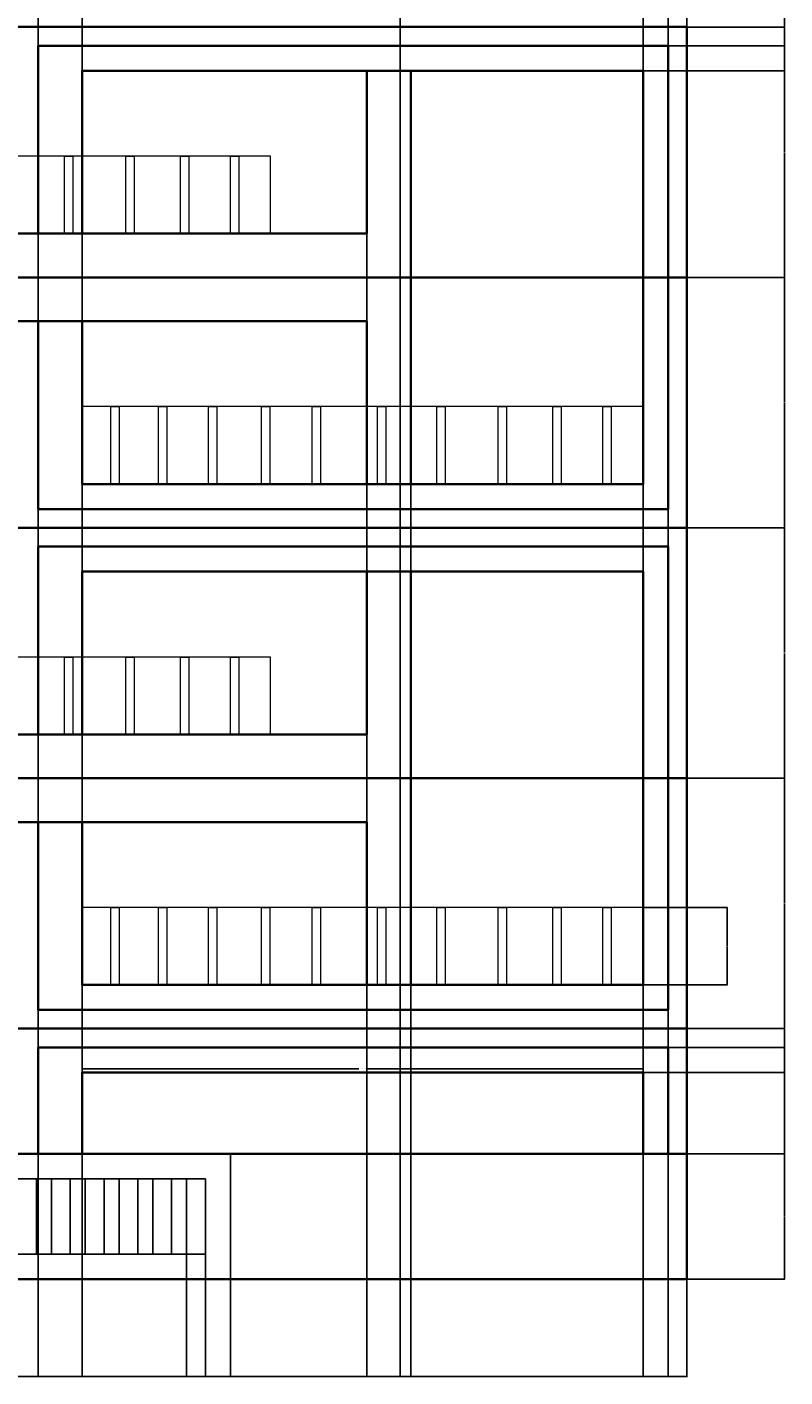
# Model space of a CAD drawing. Units: inches. Extents: x -26 to 668, y -42 to 976.
# Tile 2 of 3: x 305 to 668, y -42 to 605. Entities that reach past the tile are written whole.
import ezdxf

# ---------------------------------------------------------------- set-up
doc = ezdxf.new("R2010")
doc.units = ezdxf.units.IN
doc.header["$MEASUREMENT"] = 0
for name, color, linetype, lineweight in [('A-ANNO-DIMS', 2, 'Continuous', 18), ('A-DOOR', 3, 'Continuous', 25), ('A-ELEV', 7, 'Continuous', 35), ('A-FLOR-HRAL', 8, 'Continuous', 18)]:
    doc.layers.add(name, color=color, linetype=linetype, lineweight=lineweight)
doc.styles.get("Standard").update_dxf_attribs({"font": 'arial.ttf'})
doc.dimstyles.get("Standard").update_dxf_attribs({"dimtxt": 0.18, "dimasz": 0.18, "dimexe": 0.18, "dimexo": 0.0625, "dimgap": 0.09, "dimtad": 0, "dimtih": 1, "dimtoh": 1, "dimdec": 4, "dimzin": 0, "dimdsep": 46, "dimtxsty": 'Standard', "dimcen": 0.09, "dimadec": 0, "dimazin": 0, "dimtfac": 1, "dimtdec": 4, "dimtofl": 0, "dimtmove": 0, "dimatfit": 3, "dimfxl": 1, "dimtolj": 1, "dimtzin": 0, "dimarcsym": 0})

# ---------------------------------------------------------------- blocks, each defined once
blk = doc.blocks.new('RAILING-BALCONY')
for points in [[(331.17, 145.96), (599.79, 145.96), (599.79, 183.06), (331.17, 183.06)], [(344.86, 183.06), (348.85, 183.06), (348.85, 145.96), (344.86, 145.96)], [(367.74, 183.06), (371.72, 183.06), (371.72, 145.96), (367.74, 145.96)], [(391.66, 183.06), (395.64, 183.06), (395.64, 145.96), (391.66, 145.96)], [(417.04, 183.06), (421.03, 183.06), (421.03, 145.96), (417.04, 145.96)], [(441.38, 183.06), (445.37, 183.06), (445.37, 145.96), (441.38, 145.96)], [(472.69, 183.06), (476.68, 183.06), (476.68, 145.96), (472.69, 145.96)], [(501.02, 183.06), (505, 183.06), (505, 145.96), (501.02, 145.96)], [(530.39, 183.06), (534.38, 183.06), (534.38, 145.96), (530.39, 145.96)], [(556.62, 183.06), (560.61, 183.06), (560.61, 145.96), (556.62, 145.96)], [(580.54, 183.06), (584.53, 183.06), (584.53, 145.96), (580.54, 145.96)]]:
    blk.add_lwpolyline(points, close=True)
blk = doc.blocks.new('*D3')
at = {"layer": 'A-ANNO-DIMS', "color": 0, "lineweight": -2, "transparency": 16777216}
for p, q in [((331.17, 145.9), (331.17, 105.49)), ((599.79, 145.9), (599.79, 105.49)), ((331.35, 105.67), (463.72, 105.67)), ((599.61, 105.67), (467.25, 105.67))]:
    blk.add_line(p, q, dxfattribs=at)
at = {"layer": 'A-ANNO-DIMS', "color": 0, "transparency": 16777216}
for points in [[(331.35, 105.7), (331.35, 105.64), (331.17, 105.67)], [(599.61, 105.7), (599.61, 105.64), (599.79, 105.67)]]:
    blk.add_solid(points, dxfattribs=at)
at = {"layer": 'Defpoints', "color": 0, "transparency": 16777216}
for p in [(331.17, 145.96), (599.79, 145.96), (599.79, 105.67)]:
    blk.add_point(p, dxfattribs=at)
at = {"layer": 'A-ANNO-DIMS', "color": 0, "transparency": 16777216, "insert": (465.48, 105.67), "char_height": 0.18, "attachment_point": 5}
blk.add_mtext('\\A1;BALCONY RAILING 269 TYP.', dxfattribs=at)
blk = doc.blocks.new('*D4')
at = {"layer": 'A-ANNO-DIMS', "color": 0, "lineweight": -2, "transparency": 16777216}
for p, q in [((599.86, 183.06), (640.27, 183.06)), ((640.09, 182.88), (640.09, 164.69)), ((640.09, 146.14), (640.09, 164.33)), ((599.86, 145.96), (640.27, 145.96))]:
    blk.add_line(p, q, dxfattribs=at)
at = {"layer": 'A-ANNO-DIMS', "color": 0, "transparency": 16777216}
for points in [[(640.06, 182.88), (640.12, 182.88), (640.09, 183.06)], [(640.06, 146.14), (640.12, 146.14), (640.09, 145.96)]]:
    blk.add_solid(points, dxfattribs=at)
at = {"layer": 'Defpoints', "color": 0, "transparency": 16777216}
for p in [(599.79, 183.06), (640.09, 183.06), (599.79, 145.96)]:
    blk.add_point(p, dxfattribs=at)
at = {"layer": 'A-ANNO-DIMS', "color": 0, "transparency": 16777216, "insert": (640.09, 164.51), "char_height": 0.18, "attachment_point": 5}
blk.add_mtext('\\A1;37 TYP.', dxfattribs=at)
blk = doc.blocks.new('*D9')
at = {"layer": 'A-ANNO-DIMS', "color": 0, "lineweight": -2, "transparency": 16777216}
for p, q in [((620.86, 124.96), (667.72, 124.96)), ((667.54, 124.78), (667.54, 95.14)), ((667.54, 65.14), (667.54, 94.78)), ((620.86, 64.96), (667.72, 64.96))]:
    blk.add_line(p, q, dxfattribs=at)
at = {"layer": 'A-ANNO-DIMS', "color": 0, "transparency": 16777216}
for points in [[(667.51, 124.78), (667.57, 124.78), (667.54, 124.96)], [(667.51, 65.14), (667.57, 65.14), (667.54, 64.96)]]:
    blk.add_solid(points, dxfattribs=at)
at = {"layer": 'Defpoints', "color": 0, "transparency": 16777216}
for p in [(620.79, 124.96), (667.54, 124.96), (620.79, 64.96)]:
    blk.add_point(p, dxfattribs=at)
at = {"layer": 'A-ANNO-DIMS', "color": 0, "transparency": 16777216, "insert": (667.54, 94.96), "char_height": 0.18, "attachment_point": 5}
blk.add_mtext('\\A1;60', dxfattribs=at)
blk = doc.blocks.new('*D10')
at = {"layer": 'A-ANNO-DIMS', "color": 0, "lineweight": -2, "transparency": 16777216}
for p, q in [((620.86, 244.96), (667.72, 244.96)), ((667.54, 244.78), (667.54, 185.14)), ((667.54, 125.14), (667.54, 184.78)), ((620.86, 124.96), (667.72, 124.96))]:
    blk.add_line(p, q, dxfattribs=at)
at = {"layer": 'A-ANNO-DIMS', "color": 0, "transparency": 16777216}
for points in [[(667.51, 244.78), (667.57, 244.78), (667.54, 244.96)], [(667.51, 125.14), (667.57, 125.14), (667.54, 124.96)]]:
    blk.add_solid(points, dxfattribs=at)
at = {"layer": 'Defpoints', "color": 0, "transparency": 16777216}
for p in [(620.79, 244.96), (667.54, 244.96), (620.79, 124.96)]:
    blk.add_point(p, dxfattribs=at)
at = {"layer": 'A-ANNO-DIMS', "color": 0, "transparency": 16777216, "insert": (667.54, 184.96), "char_height": 0.18, "attachment_point": 5}
blk.add_mtext('\\A1;120', dxfattribs=at)
blk = doc.blocks.new('*D11')
at = {"layer": 'A-ANNO-DIMS', "color": 0, "lineweight": -2, "transparency": 16777216}
for p, q in [((620.86, 364.96), (667.72, 364.96)), ((667.54, 364.78), (667.54, 305.14)), ((667.54, 245.14), (667.54, 304.78)), ((620.86, 244.96), (667.72, 244.96))]:
    blk.add_line(p, q, dxfattribs=at)
at = {"layer": 'A-ANNO-DIMS', "color": 0, "transparency": 16777216}
for points in [[(667.51, 364.78), (667.57, 364.78), (667.54, 364.96)], [(667.51, 245.14), (667.57, 245.14), (667.54, 244.96)]]:
    blk.add_solid(points, dxfattribs=at)
at = {"layer": 'Defpoints', "color": 0, "transparency": 16777216}
for p in [(620.79, 364.96), (667.54, 364.96), (620.79, 244.96)]:
    blk.add_point(p, dxfattribs=at)
at = {"layer": 'A-ANNO-DIMS', "color": 0, "transparency": 16777216, "insert": (667.54, 304.96), "char_height": 0.18, "attachment_point": 5}
blk.add_mtext('\\A1;120', dxfattribs=at)
blk = doc.blocks.new('*D12')
at = {"layer": 'A-ANNO-DIMS', "color": 0, "lineweight": -2, "transparency": 16777216}
for p, q in [((620.86, 484.96), (667.72, 484.96)), ((667.54, 484.78), (667.54, 425.14)), ((667.54, 365.14), (667.54, 424.78)), ((620.86, 364.96), (667.72, 364.96))]:
    blk.add_line(p, q, dxfattribs=at)
at = {"layer": 'A-ANNO-DIMS', "color": 0, "transparency": 16777216}
for points in [[(667.51, 484.78), (667.57, 484.78), (667.54, 484.96)], [(667.51, 365.14), (667.57, 365.14), (667.54, 364.96)]]:
    blk.add_solid(points, dxfattribs=at)
at = {"layer": 'Defpoints', "color": 0, "transparency": 16777216}
for p in [(620.79, 484.96), (667.54, 484.96), (620.79, 364.96)]:
    blk.add_point(p, dxfattribs=at)
at = {"layer": 'A-ANNO-DIMS', "color": 0, "transparency": 16777216, "insert": (667.54, 424.96), "char_height": 0.18, "attachment_point": 5}
blk.add_mtext('\\A1;120', dxfattribs=at)
blk = doc.blocks.new('*D13')
at = {"layer": 'A-ANNO-DIMS', "color": 0, "lineweight": -2, "transparency": 16777216}
for p, q in [((620.86, 604.96), (667.72, 604.96)), ((667.54, 604.78), (667.54, 545.14)), ((667.54, 485.14), (667.54, 544.78)), ((620.86, 484.96), (667.72, 484.96))]:
    blk.add_line(p, q, dxfattribs=at)
at = {"layer": 'A-ANNO-DIMS', "color": 0, "transparency": 16777216}
for points in [[(667.51, 604.78), (667.57, 604.78), (667.54, 604.96)], [(667.51, 485.14), (667.57, 485.14), (667.54, 484.96)]]:
    blk.add_solid(points, dxfattribs=at)
at = {"layer": 'Defpoints', "color": 0, "transparency": 16777216}
for p in [(620.79, 604.96), (667.54, 604.96), (620.79, 484.96)]:
    blk.add_point(p, dxfattribs=at)
at = {"layer": 'A-ANNO-DIMS', "color": 0, "transparency": 16777216, "insert": (667.54, 544.96), "char_height": 0.18, "attachment_point": 5}
blk.add_mtext('\\A1;120', dxfattribs=at)
blk = doc.blocks.new('*D14')
at = {"layer": 'A-ANNO-DIMS', "color": 0, "lineweight": -2, "transparency": 16777216}
for p, q in [((620.86, 724.96), (667.72, 724.96)), ((667.54, 724.78), (667.54, 665.14)), ((667.54, 605.14), (667.54, 664.78)), ((620.86, 604.96), (667.72, 604.96))]:
    blk.add_line(p, q, dxfattribs=at)
at = {"layer": 'A-ANNO-DIMS', "color": 0, "transparency": 16777216}
for points in [[(667.51, 724.78), (667.57, 724.78), (667.54, 724.96)], [(667.51, 605.14), (667.57, 605.14), (667.54, 604.96)]]:
    blk.add_solid(points, dxfattribs=at)
at = {"layer": 'Defpoints', "color": 0, "transparency": 16777216}
for p in [(620.79, 724.96), (667.54, 724.96), (620.79, 604.96)]:
    blk.add_point(p, dxfattribs=at)
at = {"layer": 'A-ANNO-DIMS', "color": 0, "transparency": 16777216, "insert": (667.54, 664.96), "char_height": 0.18, "attachment_point": 5}
blk.add_mtext('\\A1;120', dxfattribs=at)
blk = doc.blocks.new('*D22')
at = {"layer": 'A-ANNO-DIMS', "color": 0, "lineweight": -2, "transparency": 16777216}
for p, q in [((140.65, 844.9), (140.65, -41.97)), ((483.43, 844.9), (483.43, -41.97)), ((140.83, -41.79), (311.65, -41.79)), ((483.25, -41.79), (312.43, -41.79))]:
    blk.add_line(p, q, dxfattribs=at)
at = {"layer": 'A-ANNO-DIMS', "color": 0, "transparency": 16777216}
for points in [[(140.83, -41.76), (140.83, -41.82), (140.65, -41.79)], [(483.25, -41.76), (483.25, -41.82), (483.43, -41.79)]]:
    blk.add_solid(points, dxfattribs=at)
at = {"layer": 'Defpoints', "color": 0, "transparency": 16777216}
for p in [(140.65, 844.96), (483.43, 844.96), (483.43, -41.79)]:
    blk.add_point(p, dxfattribs=at)
at = {"layer": 'A-ANNO-DIMS', "color": 0, "transparency": 16777216, "insert": (312.04, -41.79), "char_height": 0.18, "attachment_point": 5}
blk.add_mtext('\\A1;342.8', dxfattribs=at)
blk = doc.blocks.new('*D30')
at = {"layer": 'A-ANNO-DIMS', "color": 0, "lineweight": -2, "transparency": 16777216}
for p, q in [((152.83, 505.9), (152.83, -41.97)), ((310.17, 505.9), (310.17, -41.97)), ((153.01, -41.79), (231.05, -41.79)), ((309.99, -41.79), (231.96, -41.79))]:
    blk.add_line(p, q, dxfattribs=at)
at = {"layer": 'A-ANNO-DIMS', "color": 0, "transparency": 16777216}
for points in [[(153.01, -41.76), (153.01, -41.82), (152.83, -41.79)], [(309.99, -41.76), (309.99, -41.82), (310.17, -41.79)]]:
    blk.add_solid(points, dxfattribs=at)
at = {"layer": 'Defpoints', "color": 0, "transparency": 16777216}
for p in [(152.83, 505.96), (310.17, 505.96), (310.17, -41.79)]:
    blk.add_point(p, dxfattribs=at)
at = {"layer": 'A-ANNO-DIMS', "color": 0, "transparency": 16777216, "insert": (231.5, -41.79), "char_height": 0.18, "attachment_point": 5}
blk.add_mtext('\\A1;157.34', dxfattribs=at)
blk = doc.blocks.new('*D31')
at = {"layer": 'A-ANNO-DIMS', "color": 0, "lineweight": -2, "transparency": 16777216}
for p, q in [((310.17, 505.9), (310.17, -41.97)), ((331.17, 505.9), (331.17, -41.97)), ((310.35, -41.79), (320.47, -41.79)), ((330.99, -41.79), (320.87, -41.79))]:
    blk.add_line(p, q, dxfattribs=at)
at = {"layer": 'A-ANNO-DIMS', "color": 0, "transparency": 16777216}
for points in [[(310.35, -41.76), (310.35, -41.82), (310.17, -41.79)], [(330.99, -41.76), (330.99, -41.82), (331.17, -41.79)]]:
    blk.add_solid(points, dxfattribs=at)
at = {"layer": 'Defpoints', "color": 0, "transparency": 16777216}
for p in [(310.17, 505.96), (331.17, 505.96), (331.17, -41.79)]:
    blk.add_point(p, dxfattribs=at)
at = {"layer": 'A-ANNO-DIMS', "color": 0, "transparency": 16777216, "insert": (320.67, -41.79), "char_height": 0.18, "attachment_point": 5}
blk.add_mtext('\\A1;21', dxfattribs=at)
blk = doc.blocks.new('*D32')
at = {"layer": 'A-ANNO-DIMS', "color": 0, "lineweight": -2, "transparency": 16777216}
for p, q in [((331.17, 505.9), (331.17, -41.97)), ((467.51, 505.9), (467.51, -41.97)), ((331.35, -41.79), (398.88, -41.79)), ((467.33, -41.79), (399.79, -41.79))]:
    blk.add_line(p, q, dxfattribs=at)
at = {"layer": 'A-ANNO-DIMS', "color": 0, "transparency": 16777216}
for points in [[(331.35, -41.76), (331.35, -41.82), (331.17, -41.79)], [(467.33, -41.76), (467.33, -41.82), (467.51, -41.79)]]:
    blk.add_solid(points, dxfattribs=at)
at = {"layer": 'Defpoints', "color": 0, "transparency": 16777216}
for p in [(331.17, 505.96), (467.51, 505.96), (467.51, -41.79)]:
    blk.add_point(p, dxfattribs=at)
at = {"layer": 'A-ANNO-DIMS', "color": 0, "transparency": 16777216, "insert": (399.34, -41.79), "char_height": 0.18, "attachment_point": 5}
blk.add_mtext('\\A1;136.34', dxfattribs=at)
blk = doc.blocks.new('*D33')
at = {"layer": 'A-ANNO-DIMS', "color": 0, "lineweight": -2, "transparency": 16777216}
for p, q in [((488.51, 583.9), (488.51, -41.97)), ((467.51, 505.9), (467.51, -41.97)), ((467.69, -41.79), (477.8, -41.79)), ((488.33, -41.79), (478.21, -41.79))]:
    blk.add_line(p, q, dxfattribs=at)
at = {"layer": 'A-ANNO-DIMS', "color": 0, "transparency": 16777216}
for points in [[(467.69, -41.76), (467.69, -41.82), (467.51, -41.79)], [(488.33, -41.76), (488.33, -41.82), (488.51, -41.79)]]:
    blk.add_solid(points, dxfattribs=at)
at = {"layer": 'Defpoints', "color": 0, "transparency": 16777216}
for p in [(488.51, 583.96), (467.51, 505.96), (488.51, -41.79)]:
    blk.add_point(p, dxfattribs=at)
at = {"layer": 'A-ANNO-DIMS', "color": 0, "transparency": 16777216, "insert": (478.01, -41.79), "char_height": 0.18, "attachment_point": 5}
blk.add_mtext('\\A1;21', dxfattribs=at)
blk = doc.blocks.new('*D34')
at = {"layer": 'A-ANNO-DIMS', "color": 0, "lineweight": -2, "transparency": 16777216}
for p, q in [((488.51, 583.9), (488.51, -41.97)), ((599.79, 583.9), (599.79, -41.97)), ((488.69, -41.79), (543.7, -41.79)), ((599.61, -41.79), (544.61, -41.79))]:
    blk.add_line(p, q, dxfattribs=at)
at = {"layer": 'A-ANNO-DIMS', "color": 0, "transparency": 16777216}
for points in [[(488.69, -41.76), (488.69, -41.82), (488.51, -41.79)], [(599.61, -41.76), (599.61, -41.82), (599.79, -41.79)]]:
    blk.add_solid(points, dxfattribs=at)
at = {"layer": 'Defpoints', "color": 0, "transparency": 16777216}
for p in [(488.51, 583.96), (599.79, 583.96), (599.79, -41.79)]:
    blk.add_point(p, dxfattribs=at)
at = {"layer": 'A-ANNO-DIMS', "color": 0, "transparency": 16777216, "insert": (544.15, -41.79), "char_height": 0.18, "attachment_point": 5}
blk.add_mtext('\\A1;111.29', dxfattribs=at)
blk = doc.blocks.new('*D35')
at = {"layer": 'A-ANNO-DIMS', "color": 0, "lineweight": -2, "transparency": 16777216}
for p, q in [((611.79, 595.9), (611.79, -41.97)), ((599.79, 583.9), (599.79, -41.97)), ((599.97, -41.79), (605.58, -41.79)), ((611.61, -41.79), (606, -41.79))]:
    blk.add_line(p, q, dxfattribs=at)
at = {"layer": 'A-ANNO-DIMS', "color": 0, "transparency": 16777216}
for points in [[(599.97, -41.76), (599.97, -41.82), (599.79, -41.79)], [(611.61, -41.76), (611.61, -41.82), (611.79, -41.79)]]:
    blk.add_solid(points, dxfattribs=at)
at = {"layer": 'Defpoints', "color": 0, "transparency": 16777216}
for p in [(611.79, 595.96), (599.79, 583.96), (611.79, -41.79)]:
    blk.add_point(p, dxfattribs=at)
at = {"layer": 'A-ANNO-DIMS', "color": 0, "transparency": 16777216, "insert": (605.79, -41.79), "char_height": 0.18, "attachment_point": 5}
blk.add_mtext('\\A1;12', dxfattribs=at)
blk = doc.blocks.new('*D36')
at = {"layer": 'A-ANNO-DIMS', "color": 0, "lineweight": -2, "transparency": 16777216}
for p, q in [((620.79, 604.9), (620.79, -41.97)), ((611.79, 595.9), (611.79, -41.97)), ((611.97, -41.79), (616.15, -41.79)), ((620.61, -41.79), (616.44, -41.79))]:
    blk.add_line(p, q, dxfattribs=at)
at = {"layer": 'A-ANNO-DIMS', "color": 0, "transparency": 16777216}
for points in [[(611.97, -41.76), (611.97, -41.82), (611.79, -41.79)], [(620.61, -41.76), (620.61, -41.82), (620.79, -41.79)]]:
    blk.add_solid(points, dxfattribs=at)
at = {"layer": 'Defpoints', "color": 0, "transparency": 16777216}
for p in [(620.79, 604.96), (611.79, 595.96), (620.79, -41.79)]:
    blk.add_point(p, dxfattribs=at)
at = {"layer": 'A-ANNO-DIMS', "color": 0, "transparency": 16777216, "insert": (616.29, -41.79), "char_height": 0.18, "attachment_point": 5}
blk.add_mtext('\\A1;9', dxfattribs=at)
blk = doc.blocks.new('*D42')
at = {"layer": 'A-ANNO-DIMS', "color": 0, "lineweight": -2, "transparency": 16777216}
for p, q in [((611.86, 595.96), (667.72, 595.96)), ((667.54, 595.78), (667.54, 590.14)), ((667.54, 584.14), (667.54, 589.78)), ((599.86, 583.96), (667.72, 583.96))]:
    blk.add_line(p, q, dxfattribs=at)
at = {"layer": 'A-ANNO-DIMS', "color": 0, "transparency": 16777216}
for points in [[(667.51, 595.78), (667.57, 595.78), (667.54, 595.96)], [(667.51, 584.14), (667.57, 584.14), (667.54, 583.96)]]:
    blk.add_solid(points, dxfattribs=at)
at = {"layer": 'Defpoints', "color": 0, "transparency": 16777216}
for p in [(611.79, 595.96), (667.54, 595.96), (599.79, 583.96)]:
    blk.add_point(p, dxfattribs=at)
at = {"layer": 'A-ANNO-DIMS', "color": 0, "transparency": 16777216, "insert": (667.54, 589.96), "char_height": 0.18, "attachment_point": 5}
blk.add_mtext('\\A1;12', dxfattribs=at)
blk = doc.blocks.new('*D43')
at = {"layer": 'A-ANNO-DIMS', "color": 0, "lineweight": -2, "transparency": 16777216}
for p, q in [((620.86, 604.96), (667.72, 604.96)), ((667.54, 604.78), (667.54, 600.64)), ((611.86, 595.96), (667.72, 595.96)), ((667.54, 596.14), (667.54, 600.28))]:
    blk.add_line(p, q, dxfattribs=at)
at = {"layer": 'A-ANNO-DIMS', "color": 0, "transparency": 16777216}
for points in [[(667.51, 604.78), (667.57, 604.78), (667.54, 604.96)], [(667.51, 596.14), (667.57, 596.14), (667.54, 595.96)]]:
    blk.add_solid(points, dxfattribs=at)
at = {"layer": 'Defpoints', "color": 0, "transparency": 16777216}
for p in [(620.79, 604.96), (667.54, 604.96), (611.79, 595.96)]:
    blk.add_point(p, dxfattribs=at)
at = {"layer": 'A-ANNO-DIMS', "color": 0, "transparency": 16777216, "insert": (667.54, 600.46), "char_height": 0.18, "attachment_point": 5}
blk.add_mtext('\\A1;9', dxfattribs=at)
blk = doc.blocks.new('*D44')
at = {"layer": 'A-ANNO-DIMS', "color": 0, "lineweight": -2, "transparency": 16777216}
for p, q in [((611.86, 613.96), (667.72, 613.96)), ((667.54, 613.78), (667.54, 609.64)), ((667.54, 605.14), (667.54, 609.28)), ((620.86, 604.96), (667.72, 604.96))]:
    blk.add_line(p, q, dxfattribs=at)
at = {"layer": 'A-ANNO-DIMS', "color": 0, "transparency": 16777216}
for points in [[(667.51, 613.78), (667.57, 613.78), (667.54, 613.96)], [(667.51, 605.14), (667.57, 605.14), (667.54, 604.96)]]:
    blk.add_solid(points, dxfattribs=at)
at = {"layer": 'Defpoints', "color": 0, "transparency": 16777216}
for p in [(611.79, 613.96), (667.54, 613.96), (620.79, 604.96)]:
    blk.add_point(p, dxfattribs=at)
at = {"layer": 'A-ANNO-DIMS', "color": 0, "transparency": 16777216, "insert": (667.54, 609.46), "char_height": 0.18, "attachment_point": 5}
blk.add_mtext('\\A1;9', dxfattribs=at)
blk = doc.blocks.new('*D55')
at = {"layer": 'A-ANNO-DIMS', "color": 0, "lineweight": -2, "transparency": 16777216}
for p, q in [((293.12, 16.9), (293.12, -41.97)), ((381.21, 16.9), (381.21, -41.97)), ((293.3, -41.79), (336.86, -41.79)), ((381.03, -41.79), (337.47, -41.79))]:
    blk.add_line(p, q, dxfattribs=at)
at = {"layer": 'A-ANNO-DIMS', "color": 0, "transparency": 16777216}
for points in [[(293.3, -41.76), (293.3, -41.82), (293.12, -41.79)], [(381.03, -41.76), (381.03, -41.82), (381.21, -41.79)]]:
    blk.add_solid(points, dxfattribs=at)
at = {"layer": 'Defpoints', "color": 0, "transparency": 16777216}
for p in [(293.12, 16.96), (381.21, 16.96), (381.21, -41.79)]:
    blk.add_point(p, dxfattribs=at)
at = {"layer": 'A-ANNO-DIMS', "color": 0, "transparency": 16777216, "insert": (337.16, -41.79), "char_height": 0.18, "attachment_point": 5}
blk.add_mtext('\\A1;88.1', dxfattribs=at)
blk = doc.blocks.new('*D56')
at = {"layer": 'A-ANNO-DIMS', "color": 0, "lineweight": -2, "transparency": 16777216}
for p, q in [((381.21, 16.9), (381.21, -41.97)), ((390.22, 16.9), (390.22, -41.97)), ((381.39, -41.79), (385.32, -41.79)), ((390.04, -41.79), (386.11, -41.79))]:
    blk.add_line(p, q, dxfattribs=at)
at = {"layer": 'A-ANNO-DIMS', "color": 0, "transparency": 16777216}
for points in [[(381.39, -41.76), (381.39, -41.82), (381.21, -41.79)], [(390.04, -41.76), (390.04, -41.82), (390.22, -41.79)]]:
    blk.add_solid(points, dxfattribs=at)
at = {"layer": 'Defpoints', "color": 0, "transparency": 16777216}
for p in [(381.21, 16.96), (390.22, 16.96), (390.22, -41.79)]:
    blk.add_point(p, dxfattribs=at)
at = {"layer": 'A-ANNO-DIMS', "color": 0, "transparency": 16777216, "insert": (385.72, -41.79), "char_height": 0.18, "attachment_point": 5}
blk.add_mtext('\\A1;9.007', dxfattribs=at)
blk = doc.blocks.new('*D57')
at = {"layer": 'A-ANNO-DIMS', "color": 0, "lineweight": -2, "transparency": 16777216}
for p, q in [((390.22, 16.9), (390.22, -41.97)), ((402.22, 4.9), (402.22, -41.97)), ((390.4, -41.79), (396.01, -41.79)), ((402.04, -41.79), (396.43, -41.79))]:
    blk.add_line(p, q, dxfattribs=at)
at = {"layer": 'A-ANNO-DIMS', "color": 0, "transparency": 16777216}
for points in [[(390.4, -41.76), (390.4, -41.82), (390.22, -41.79)], [(402.04, -41.76), (402.04, -41.82), (402.22, -41.79)]]:
    blk.add_solid(points, dxfattribs=at)
at = {"layer": 'Defpoints', "color": 0, "transparency": 16777216}
for p in [(390.22, 16.96), (402.22, 4.96), (402.22, -41.79)]:
    blk.add_point(p, dxfattribs=at)
at = {"layer": 'A-ANNO-DIMS', "color": 0, "transparency": 16777216, "insert": (396.22, -41.79), "char_height": 0.18, "attachment_point": 5}
blk.add_mtext('\\A1;12', dxfattribs=at)
blk = doc.blocks.new('*D58')
at = {"layer": 'A-ANNO-DIMS', "color": 0, "lineweight": -2, "transparency": 16777216}
for p, q in [((402.22, 4.9), (402.22, -41.97)), ((620.79, 4.9), (620.79, -41.97)), ((402.4, -41.79), (511.04, -41.79)), ((620.61, -41.79), (511.97, -41.79))]:
    blk.add_line(p, q, dxfattribs=at)
at = {"layer": 'A-ANNO-DIMS', "color": 0, "transparency": 16777216}
for points in [[(402.4, -41.76), (402.4, -41.82), (402.22, -41.79)], [(620.61, -41.76), (620.61, -41.82), (620.79, -41.79)]]:
    blk.add_solid(points, dxfattribs=at)
at = {"layer": 'Defpoints', "color": 0, "transparency": 16777216}
for p in [(402.22, 4.96), (620.79, 4.96), (620.79, -41.79)]:
    blk.add_point(p, dxfattribs=at)
at = {"layer": 'A-ANNO-DIMS', "color": 0, "transparency": 16777216, "insert": (511.51, -41.79), "char_height": 0.18, "attachment_point": 5}
blk.add_mtext('\\A1;218.57', dxfattribs=at)
blk = doc.blocks.new('*D62')
at = {"layer": 'A-ANNO-DIMS', "color": 0, "lineweight": -2, "transparency": 16777216}
for p, q in [((620.86, 64.96), (667.72, 64.96)), ((667.54, 64.78), (667.54, 35.14)), ((667.54, 5.14), (667.54, 34.78)), ((620.86, 4.96), (667.72, 4.96))]:
    blk.add_line(p, q, dxfattribs=at)
at = {"layer": 'A-ANNO-DIMS', "color": 0, "transparency": 16777216}
for points in [[(667.51, 64.78), (667.57, 64.78), (667.54, 64.96)], [(667.51, 5.14), (667.57, 5.14), (667.54, 4.96)]]:
    blk.add_solid(points, dxfattribs=at)
at = {"layer": 'Defpoints', "color": 0, "transparency": 16777216}
for p in [(620.79, 64.96), (667.54, 64.96), (620.79, 4.96)]:
    blk.add_point(p, dxfattribs=at)
at = {"layer": 'A-ANNO-DIMS', "color": 0, "transparency": 16777216, "insert": (667.54, 34.96), "char_height": 0.18, "attachment_point": 5}
blk.add_mtext('\\A1;60', dxfattribs=at)
blk = doc.blocks.new('*D63')
at = {"layer": 'A-ANNO-DIMS', "color": 0, "lineweight": -2, "transparency": 16777216}
for p, q in [((599.86, 103.96), (667.72, 103.96)), ((667.54, 103.78), (667.54, 84.64)), ((667.54, 65.14), (667.54, 84.28)), ((620.86, 64.96), (667.72, 64.96))]:
    blk.add_line(p, q, dxfattribs=at)
at = {"layer": 'A-ANNO-DIMS', "color": 0, "transparency": 16777216}
for points in [[(667.51, 103.78), (667.57, 103.78), (667.54, 103.96)], [(667.51, 65.14), (667.57, 65.14), (667.54, 64.96)]]:
    blk.add_solid(points, dxfattribs=at)
at = {"layer": 'Defpoints', "color": 0, "transparency": 16777216}
for p in [(599.79, 103.96), (667.54, 103.96), (620.79, 64.96)]:
    blk.add_point(p, dxfattribs=at)
at = {"layer": 'A-ANNO-DIMS', "color": 0, "transparency": 16777216, "insert": (667.54, 84.46), "char_height": 0.18, "attachment_point": 5}
blk.add_mtext('\\A1;39', dxfattribs=at)
blk = doc.blocks.new('*D64')
at = {"layer": 'A-ANNO-DIMS', "color": 0, "lineweight": -2, "transparency": 16777216}
for p, q in [((611.86, 115.96), (667.72, 115.96)), ((667.54, 115.78), (667.54, 110.14)), ((599.86, 103.96), (667.72, 103.96)), ((667.54, 104.14), (667.54, 109.78))]:
    blk.add_line(p, q, dxfattribs=at)
at = {"layer": 'A-ANNO-DIMS', "color": 0, "transparency": 16777216}
for points in [[(667.51, 115.78), (667.57, 115.78), (667.54, 115.96)], [(667.51, 104.14), (667.57, 104.14), (667.54, 103.96)]]:
    blk.add_solid(points, dxfattribs=at)
at = {"layer": 'Defpoints', "color": 0, "transparency": 16777216}
for p in [(611.79, 115.96), (667.54, 115.96), (599.79, 103.96)]:
    blk.add_point(p, dxfattribs=at)
at = {"layer": 'A-ANNO-DIMS', "color": 0, "transparency": 16777216, "insert": (667.54, 109.96), "char_height": 0.18, "attachment_point": 5}
blk.add_mtext('\\A1;12', dxfattribs=at)
blk = doc.blocks.new('*D66')
at = {"layer": 'A-ANNO-DIMS', "color": 0, "lineweight": -2, "transparency": 16777216}
for p, q in [((310.17, 65.02), (310.17, 975.89)), ((310.35, 975.71), (320.47, 975.71)), ((330.99, 975.71), (320.87, 975.71)), ((331.17, 65.02), (331.17, 975.89))]:
    blk.add_line(p, q, dxfattribs=at)
at = {"layer": 'A-ANNO-DIMS', "color": 0, "transparency": 16777216}
for points in [[(310.35, 975.74), (310.35, 975.68), (310.17, 975.71)], [(330.99, 975.74), (330.99, 975.68), (331.17, 975.71)]]:
    blk.add_solid(points, dxfattribs=at)
at = {"layer": 'Defpoints', "color": 0, "transparency": 16777216}
for p in [(331.17, 975.71), (310.17, 64.96), (331.17, 64.96)]:
    blk.add_point(p, dxfattribs=at)
at = {"layer": 'A-ANNO-DIMS', "color": 0, "transparency": 16777216, "insert": (320.67, 975.71), "char_height": 0.18, "attachment_point": 5}
blk.add_mtext('\\A1;21', dxfattribs=at)
blk = doc.blocks.new('*D67')
at = {"layer": 'A-ANNO-DIMS', "color": 0, "lineweight": -2, "transparency": 16777216}
for p, q in [((331.17, 65.02), (331.17, 975.89)), ((331.35, 975.71), (465.09, 975.71)), ((599.61, 975.71), (465.88, 975.71)), ((599.79, 65.02), (599.79, 975.89))]:
    blk.add_line(p, q, dxfattribs=at)
at = {"layer": 'A-ANNO-DIMS', "color": 0, "transparency": 16777216}
for points in [[(331.35, 975.74), (331.35, 975.68), (331.17, 975.71)], [(599.61, 975.74), (599.61, 975.68), (599.79, 975.71)]]:
    blk.add_solid(points, dxfattribs=at)
at = {"layer": 'Defpoints', "color": 0, "transparency": 16777216}
for p in [(599.79, 975.71), (331.17, 64.96), (599.79, 64.96)]:
    blk.add_point(p, dxfattribs=at)
at = {"layer": 'A-ANNO-DIMS', "color": 0, "transparency": 16777216, "insert": (465.48, 975.71), "char_height": 0.18, "attachment_point": 5}
blk.add_mtext('\\A1;268.6', dxfattribs=at)
blk = doc.blocks.new('*D68')
at = {"layer": 'A-ANNO-DIMS', "color": 0, "lineweight": -2, "transparency": 16777216}
for p, q in [((599.79, 65.02), (599.79, 975.89)), ((599.97, 975.71), (605.58, 975.71)), ((611.61, 975.71), (606, 975.71)), ((611.79, 65.02), (611.79, 975.89))]:
    blk.add_line(p, q, dxfattribs=at)
at = {"layer": 'A-ANNO-DIMS', "color": 0, "transparency": 16777216}
for points in [[(599.97, 975.74), (599.97, 975.68), (599.79, 975.71)], [(611.61, 975.74), (611.61, 975.68), (611.79, 975.71)]]:
    blk.add_solid(points, dxfattribs=at)
at = {"layer": 'Defpoints', "color": 0, "transparency": 16777216}
for p in [(611.79, 975.71), (599.79, 64.96), (611.79, 64.96)]:
    blk.add_point(p, dxfattribs=at)
at = {"layer": 'A-ANNO-DIMS', "color": 0, "transparency": 16777216, "insert": (605.79, 975.71), "char_height": 0.18, "attachment_point": 5}
blk.add_mtext('\\A1;12', dxfattribs=at)
blk = doc.blocks.new('*D69')
at = {"layer": 'A-ANNO-DIMS', "color": 0, "lineweight": -2, "transparency": 16777216}
for p, q in [((611.79, 65.02), (611.79, 975.89)), ((611.97, 975.71), (616.15, 975.71)), ((620.61, 975.71), (616.44, 975.71)), ((620.79, 65.02), (620.79, 975.89))]:
    blk.add_line(p, q, dxfattribs=at)
at = {"layer": 'A-ANNO-DIMS', "color": 0, "transparency": 16777216}
for points in [[(611.97, 975.74), (611.97, 975.68), (611.79, 975.71)], [(620.61, 975.74), (620.61, 975.68), (620.79, 975.71)]]:
    blk.add_solid(points, dxfattribs=at)
at = {"layer": 'Defpoints', "color": 0, "transparency": 16777216}
for p in [(620.79, 975.71), (611.79, 64.96), (620.79, 64.96)]:
    blk.add_point(p, dxfattribs=at)
at = {"layer": 'A-ANNO-DIMS', "color": 0, "transparency": 16777216, "insert": (616.29, 975.71), "char_height": 0.18, "attachment_point": 5}
blk.add_mtext('\\A1;9', dxfattribs=at)

msp = doc.modelspace()

# ---------------------------------------------------------------- linework, layer by layer
at = {"layer": 'A-DOOR'}
for points in [[(149.7506, 64.9609), (402.2206, 64.9609), (402.2206, 4.9609), (149.7506, 4.9609)], [(161.7506, 52.9609), (390.2206, 52.9609), (390.2206, 16.9609), (161.7506, 16.9609)], [(316.4764, 16.9609), (309.2994, 16.9609), (309.2994, 52.9609), (316.4764, 52.9609)], [(332.6607, 16.9609), (325.4836, 16.9609), (325.4836, 52.9609), (332.6607, 52.9609)], [(348.8449, 16.9609), (341.6679, 16.9609), (341.6679, 52.9609), (348.8449, 52.9609)], [(365.0292, 16.9609), (357.8521, 16.9609), (357.8521, 52.9609), (365.0292, 52.9609)], [(381.2134, 16.9609), (374.0364, 16.9609), (374.0364, 52.9609), (381.2134, 52.9609)]]:
    msp.add_lwpolyline(points, close=True, dxfattribs=at)
at = {"layer": 'A-ELEV'}
for p, q in [((310.1714, 133.9609), (479.5079, 133.9609)), ((620.7944, 124.9609), (131.8349, 124.9609)), ((620.7944, 4.9609), (620.7944, 124.9609)), ((20.7944, 64.9609), (620.7944, 64.9609)), ((20.7944, 4.9609), (620.7944, 4.9609))]:
    msp.add_line(p, q, dxfattribs=at)
for points in [[(131.8349, 484.9609), (620.7944, 484.9609), (620.7944, 604.9609), (131.8349, 604.9609)], [(331.1714, 505.9609), (152.8349, 505.9609), (152.8349, 595.9609)], [(310.1714, 505.9609), (310.1714, 595.9609)], [(310.1714, 595.9609), (611.7944, 595.9609), (611.7944, 484.9609)], [(331.1714, 583.9609), (467.5079, 583.9609), (467.5079, 505.9609), (331.1714, 505.9609)], [(467.5079, 505.9609), (331.1714, 505.9609), (331.1714, 583.9609), (599.7944, 583.9609), (599.7944, 484.9609)], [(488.5079, 583.9609), (488.5079, 484.9609)], [(131.8349, 364.9609), (620.7944, 364.9609), (620.7944, 484.9609), (131.8349, 484.9609)], [(319.1714, 373.9609), (611.7944, 373.9609), (611.7944, 484.9609)], [(467.5079, 463.9609), (331.1714, 463.9609), (331.1714, 385.9609), (599.7944, 385.9609), (599.7944, 484.9609)], [(488.5079, 385.9609), (488.5079, 484.9609)], [(331.1714, 463.9609), (152.8349, 463.9609), (152.8349, 373.9609)], [(310.1714, 463.9609), (310.1714, 373.9609)], [(331.1714, 385.9609), (467.5079, 385.9609), (467.5079, 463.9609), (331.1714, 463.9609)], [(310.1714, 373.9609), (479.5079, 373.9609)], [(131.8349, 244.9609), (620.7944, 244.9609), (620.7944, 364.9609), (131.8349, 364.9609)], [(131.8349, 244.9609), (131.8349, 364.9609), (504.2381, 364.9609)], [(331.1714, 265.9609), (152.8349, 265.9609), (152.8349, 355.9609)], [(310.1714, 265.9609), (310.1714, 355.9609)], [(310.1714, 355.9609), (611.7944, 355.9609), (611.7944, 244.9609)], [(331.1714, 343.9609), (467.5079, 343.9609), (467.5079, 265.9609), (331.1714, 265.9609)], [(467.5079, 265.9609), (331.1714, 265.9609), (331.1714, 343.9609), (599.7944, 343.9609), (599.7944, 244.9609)], [(488.5079, 343.9609), (488.5079, 244.9609)], [(131.8349, 124.9609), (620.7944, 124.9609), (620.7944, 244.9609), (131.8349, 244.9609)], [(504.2381, 124.9609), (131.8349, 124.9609), (131.8349, 244.9609), (504.2381, 244.9609)], [(488.5079, 244.9609), (131.8349, 244.9609), (131.8349, 124.9609), (488.5079, 124.9609)], [(310.1714, 124.9609), (620.7944, 124.9609), (620.7944, 244.9609), (310.1714, 244.9609)], [(318.0365, 244.9609), (620.7944, 244.9609), (620.7944, 124.9609), (318.0365, 124.9609)], [(319.1714, 133.9609), (611.7944, 133.9609), (611.7944, 244.9609)], [(467.5079, 223.9609), (331.1714, 223.9609), (331.1714, 145.9609), (599.7944, 145.9609), (599.7944, 244.9609)], [(488.5079, 145.9609), (488.5079, 244.9609)], [(331.1714, 223.9609), (152.8349, 223.9609), (152.8349, 133.9609)], [(310.1714, 223.9609), (310.1714, 133.9609)], [(331.1714, 145.9609), (467.5079, 145.9609), (467.5079, 223.9609), (331.1714, 223.9609)], [(310.1714, 64.9609), (310.1714, 115.9609)], [(310.1714, 115.9609), (611.7944, 115.9609), (611.7944, 64.9609)], [(331.1714, 64.9609), (331.1714, 103.9609), (599.7944, 103.9609), (599.7944, 64.9609)]]:
    msp.add_lwpolyline(points, dxfattribs=at)

# ---------------------------------------------------------------- block references
at = {"layer": 'A-FLOR-HRAL'}
for p in [(-178.3365, 360), (0, 240), (-178.3365, 120), (0, 0)]:
    msp.add_blockref('RAILING-BALCONY', p, dxfattribs=at)

# ---------------------------------------------------------------- dimensions: what is measured, and where the dimension line sits
at = {"layer": 'A-ANNO-DIMS'}
for base, p1, p2, override, picture, middle in [((331.1714, 975.7109), (310.1714, 64.9609), (331.1714, 64.9609), {"dimdec": 0, "dimlfac": 1, "dimrnd": 0, "dimzin": 0, "dimdsep": 46, "dimlunit": 2}, '*D66', (320.6714, 975.7109)), ((599.7944, 975.7109), (331.1714, 64.9609), (599.7944, 64.9609), {"dimdec": 1, "dimlfac": 1, "dimrnd": 0, "dimzin": 0, "dimdsep": 46, "dimlunit": 2}, '*D67', (465.4829, 975.7109)), ((611.7944, 975.7109), (599.7944, 64.9609), (611.7944, 64.9609), {"dimdec": 0, "dimlfac": 1, "dimrnd": 0, "dimzin": 0, "dimdsep": 46, "dimlunit": 2}, '*D68', (605.7944, 975.7109)), ((620.7944, 975.7109), (611.7944, 64.9609), (620.7944, 64.9609), {"dimdec": 0, "dimlfac": 1, "dimrnd": 0, "dimzin": 0, "dimdsep": 46, "dimlunit": 2}, '*D69', (616.2944, 975.7109)), ((483.4325, -41.7891), (140.6477, 844.9609), (483.4325, 844.9609), {"dimdec": 1, "dimlfac": 1, "dimrnd": 0, "dimzin": 0, "dimdsep": 46, "dimlunit": 2}, '*D22', (312.0401, -41.7891)), ((620.7944, -41.7891), (611.7944, 595.9609), (620.7944, 604.9609), {"dimdec": 0, "dimlfac": 1, "dimrnd": 0, "dimzin": 0, "dimdsep": 46, "dimlunit": 2}, '*D36', (616.2944, -41.7891)), ((611.7944, -41.7891), (599.7944, 583.9609), (611.7944, 595.9609), {"dimdec": 0, "dimlfac": 1, "dimrnd": 0, "dimzin": 0, "dimdsep": 46, "dimlunit": 2}, '*D35', (605.7944, -41.7891)), ((488.5079, -41.7891), (467.5079, 505.9609), (488.5079, 583.9609), {"dimdec": 0, "dimlfac": 1, "dimrnd": 0, "dimzin": 0, "dimdsep": 46, "dimlunit": 2}, '*D33', (478.0079, -41.7891)), ((599.7944, -41.7891), (488.5079, 583.9609), (599.7944, 583.9609), {"dimdec": 2, "dimlfac": 1, "dimrnd": 0, "dimzin": 0, "dimdsep": 46, "dimlunit": 2}, '*D34', (544.1511, -41.7891)), ((310.1714, -41.7891), (152.8349, 505.9609), (310.1714, 505.9609), {"dimdec": 2, "dimlfac": 1, "dimrnd": 0, "dimzin": 0, "dimdsep": 46, "dimlunit": 2}, '*D30', (231.5031, -41.7891)), ((331.1714, -41.7891), (310.1714, 505.9609), (331.1714, 505.9609), {"dimdec": 0, "dimlfac": 1, "dimrnd": 0, "dimzin": 0, "dimdsep": 46, "dimlunit": 2}, '*D31', (320.6714, -41.7891)), ((467.5079, -41.7891), (331.1714, 505.9609), (467.5079, 505.9609), {"dimdec": 2, "dimlfac": 1, "dimrnd": 0, "dimzin": 0, "dimdsep": 46, "dimlunit": 2}, '*D32', (399.3396, -41.7891)), ((381.2134, -41.7891), (293.1151, 16.9609), (381.2134, 16.9609), {"dimdec": 1, "dimlfac": 1, "dimrnd": 0, "dimzin": 0, "dimdsep": 46, "dimlunit": 2}, '*D55', (337.1643, -41.7891)), ((390.2206, -41.7891), (381.2134, 16.9609), (390.2206, 16.9609), {"dimdec": 3, "dimlfac": 1, "dimrnd": 0, "dimzin": 0, "dimdsep": 46, "dimlunit": 2}, '*D56', (385.717, -41.7891)), ((402.2206, -41.7891), (390.2206, 16.9609), (402.2206, 4.9609), {"dimdec": 0, "dimlfac": 1, "dimrnd": 0, "dimzin": 0, "dimdsep": 46, "dimlunit": 2}, '*D57', (396.2206, -41.7891)), ((620.7944, -41.7891), (402.2206, 4.9609), (620.7944, 4.9609), {"dimdec": 2, "dimlfac": 1, "dimrnd": 0, "dimzin": 0, "dimdsep": 46, "dimlunit": 2}, '*D58', (511.5075, -41.7891))]:
    dim = msp.add_linear_dim(base=base, p1=p1, p2=p2, dimstyle='Standard', override=override, dxfattribs=at)
    dim.commit()
    dim.dimension.update_dxf_attribs({"geometry": picture, "text_midpoint": middle})
for base, p1, p2, picture, middle in [((667.5444, 724.9609), (620.7944, 604.9609), (620.7944, 724.9609), '*D14', (667.5444, 664.9609)), ((667.5444, 613.9609), (620.7944, 604.9609), (611.7944, 613.9609), '*D44', (667.5444, 609.4609)), ((667.5444, 604.9609), (611.7944, 595.9609), (620.7944, 604.9609), '*D43', (667.5444, 600.4609)), ((667.5444, 604.9609), (620.7944, 484.9609), (620.7944, 604.9609), '*D13', (667.5444, 544.9609)), ((667.5444, 595.9609), (599.7944, 583.9609), (611.7944, 595.9609), '*D42', (667.5444, 589.9609)), ((667.5444, 484.9609), (620.7944, 364.9609), (620.7944, 484.9609), '*D12', (667.5444, 424.9609)), ((667.5444, 364.9609), (620.7944, 244.9609), (620.7944, 364.9609), '*D11', (667.5444, 304.9609)), ((667.5444, 244.9609), (620.7944, 124.9609), (620.7944, 244.9609), '*D10', (667.5444, 184.9609)), ((667.5444, 124.9609), (620.7944, 64.9609), (620.7944, 124.9609), '*D9', (667.5444, 94.9609)), ((667.5444, 115.9609), (599.7944, 103.9609), (611.7944, 115.9609), '*D64', (667.5444, 109.9609)), ((667.5444, 103.9609), (620.7944, 64.9609), (599.7944, 103.9609), '*D63', (667.5444, 84.4609)), ((667.5444, 64.9609), (620.7944, 4.9609), (620.7944, 64.9609), '*D62', (667.5444, 34.9609))]:
    dim = msp.add_linear_dim(base=base, p1=p1, p2=p2, angle=90, dimstyle='Standard', override={"dimdec": 0, "dimlfac": 1, "dimrnd": 0, "dimzin": 0, "dimdsep": 46, "dimlunit": 2}, dxfattribs=at)
    dim.commit()
    dim.dimension.update_dxf_attribs({"geometry": picture, "text_midpoint": middle})
dim = msp.add_linear_dim(base=(640.0878, 183.0553), p1=(599.7944, 145.9609), p2=(599.7944, 183.0553), angle=90, text='<> TYP.', dimstyle='Standard', override={"dimdec": 0, "dimlfac": 1, "dimrnd": 0, "dimzin": 0, "dimdsep": 46, "dimlunit": 2}, dxfattribs=at)
dim.commit()
dim.dimension.update_dxf_attribs({"geometry": '*D4', "text_midpoint": (640.0878, 164.5081)})
dim = msp.add_linear_dim(base=(599.7944, 105.6674), p1=(331.1714, 145.9609), p2=(599.7944, 145.9609), text='BALCONY RAILING <> TYP.', dimstyle='Standard', override={"dimdec": 0, "dimlfac": 1, "dimrnd": 0, "dimzin": 0, "dimdsep": 46, "dimlunit": 2}, dxfattribs=at)
dim.commit()
dim.dimension.update_dxf_attribs({"geometry": '*D3', "text_midpoint": (465.4829, 105.6674)})

doc.saveas('drawing.dxf')
